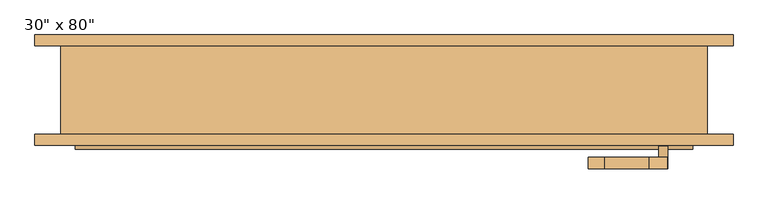
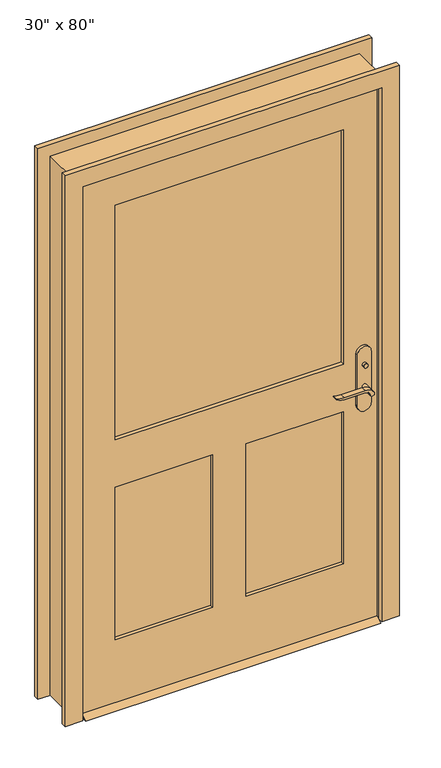
"""IFC4 building model written with IfcOpenShell, lengths in millimetres: door geometry."""

from ifc_helpers import new_model, si_unit, point, frame, frame_2d, origin, place, context, project, spatial, polyline, circle_curve, trimmed, segment, composite_curve, outline, extrude, faceted_brep, source, transform, mapped, element, save


def door_f970b2d0(model_context):
    return source(origin(), model_context, "Body", "SolidModel", [
        extrude(outline(polyline([(-38.1, 12.7), (-12.7, 0.0), (-98.425, 0.0), (-73.025, 12.7), (-38.1, 12.7)])), frame((-533.4, 0.0, 0.0), z_axis=(1.0, 0.0, 0.0), x_axis=(0.0, 1.0, 0.0)), (0.0, 0.0, 1.0), 1066.8),
        extrude(outline(polyline([(487.6, -18.1), (487.6, -28.1), (477.6, -28.1), (477.6, -18.1), (487.6, -18.1)])), frame((0.0, 0.0, 981.9), z_axis=(0.0, 0.0, 1.0), x_axis=(1.0, 0.0, 0.0)), (0.0, 0.0, 1.0), 30.0),
        extrude(outline(composite_curve([segment(trimmed(circle_curve(frame_2d((996.9, 482.6)), 8.0), [point((996.9, 474.6))], [point((996.9, 490.6))], False, "CARTESIAN"), True, "CONTINUOUS"), segment(trimmed(circle_curve(frame_2d((996.9, 482.6)), 8.0), [point((996.9, 490.6))], [point((996.9, 474.6))], False, "CARTESIAN"), True, "CONTINUOUS")], self_intersect=False)), frame((0.0, -93.025, 0.0), z_axis=(0.0, 1.0, 0.0), x_axis=(0.0, 0.0, 1.0)), (0.0, 0.0, 1.0), 10.0),
        extrude(outline(composite_curve([segment(trimmed(circle_curve(frame_2d((897.1555521, 458.9324871)), 37.2832219), [point((919.0523287, 489.1081363))], [point((934.4, 457.2325667))], False, "CARTESIAN"), True, "CONTINUOUS"), segment(polyline([(934.4, 457.2325667), (934.4, 380.9564091)]), True, "CONTINUOUS"), segment(trimmed(circle_curve(frame_2d((1017.6850638, 381.0227909)), 83.2850902), [point((934.4, 380.9564091))], [point((939.4, 352.6))], True, "CARTESIAN"), True, "CONTINUOUS"), segment(polyline([(939.4, 352.6), (936.6135558, 352.6)]), True, "CONTINUOUS"), segment(trimmed(circle_curve(frame_2d((986.6709207, 384.5396612)), 59.3791355), [point((936.6135558, 352.6))], [point((927.4, 380.9564091))], False, "CARTESIAN"), True, "CONTINUOUS"), segment(polyline([(927.4, 380.9564091), (927.4, 457.2138099)]), True, "CONTINUOUS"), segment(trimmed(circle_curve(frame_2d((909.2738613, 457.2138099)), 18.1261387), [point((927.4, 457.2138099))], [point((914.4, 474.6))], True, "CARTESIAN"), True, "CONTINUOUS"), segment(trimmed(circle_curve(frame_2d((914.4, 482.6)), 8.0), [point((914.4, 474.6))], [point((919.0523287, 489.1081363))], False, "CARTESIAN"), True, "CONTINUOUS")], self_intersect=False)), frame((0.0, 1.9, 0.0), z_axis=(0.0, 1.0, 0.0), x_axis=(0.0, 0.0, 1.0)), (0.0, 0.0, 1.0), 20.0),
        extrude(outline(composite_curve([segment(trimmed(circle_curve(frame_2d((914.4, 482.6)), 8.0), [point((914.3999903, 474.6))], [point((919.0523287, 489.1081363))], False, "CARTESIAN"), True, "CONTINUOUS"), segment(trimmed(circle_curve(frame_2d((897.1555521, 458.9324871)), 37.2832219), [point((919.0523287, 489.1081363))], [point((934.4, 457.2325667))], False, "CARTESIAN"), True, "CONTINUOUS"), segment(polyline([(934.4, 457.2325667), (934.4, 380.9564091)]), True, "CONTINUOUS"), segment(trimmed(circle_curve(frame_2d((1017.6850638, 381.0227909)), 83.2850902), [point((934.4, 380.9564091))], [point((939.4, 352.6))], True, "CARTESIAN"), True, "CONTINUOUS"), segment(polyline([(939.4, 352.6), (936.6135558, 352.6)]), True, "CONTINUOUS"), segment(trimmed(circle_curve(frame_2d((986.6709207, 384.5396612)), 59.3791355), [point((936.6135558, 352.6))], [point((927.4, 380.9564091))], False, "CARTESIAN"), True, "CONTINUOUS"), segment(polyline([(927.4, 380.9564091), (927.4, 457.2138122)]), True, "CONTINUOUS"), segment(trimmed(circle_curve(frame_2d((909.2738682, 457.2138122)), 18.1261318), [point((927.4, 457.2138122))], [point((914.3999903, 474.6))], True, "CARTESIAN"), True, "CONTINUOUS")], self_intersect=False)), frame((0.0, -133.025, 0.0), z_axis=(0.0, 1.0, 0.0), x_axis=(0.0, 0.0, 1.0)), (0.0, 0.0, 1.0), 20.0),
        extrude(outline(composite_curve([segment(trimmed(circle_curve(frame_2d((914.4, 482.6)), 8.0), [point((914.4, 474.6))], [point((914.4, 490.6))], False, "CARTESIAN"), True, "CONTINUOUS"), segment(trimmed(circle_curve(frame_2d((914.4, 482.6)), 8.0), [point((914.4, 490.6))], [point((914.4, 474.6))], False, "CARTESIAN"), True, "CONTINUOUS")], self_intersect=False)), frame((0.0, -28.1, 0.0), z_axis=(0.0, 1.0, 0.0), x_axis=(0.0, 0.0, 1.0)), (0.0, 0.0, 1.0), 30.0),
        extrude(outline(composite_curve([segment(trimmed(circle_curve(frame_2d((914.4, 482.6)), 8.0), [point((914.4, 474.6))], [point((914.4, 490.6))], False, "CARTESIAN"), True, "CONTINUOUS"), segment(trimmed(circle_curve(frame_2d((914.4, 482.6)), 8.0), [point((914.4, 490.6))], [point((914.4, 474.6))], False, "CARTESIAN"), True, "CONTINUOUS")], self_intersect=False)), frame((0.0, -113.025, 0.0), z_axis=(0.0, 1.0, 0.0), x_axis=(0.0, 0.0, 1.0)), (0.0, 0.0, 1.0), 30.0),
        extrude(outline(composite_curve([segment(polyline([(844.4, 507.6), (1039.4, 507.6)]), True, "CONTINUOUS"), segment(trimmed(circle_curve(frame_2d((1039.4, 482.6)), 25.0), [point((1039.4, 507.6))], [point((1039.4, 457.6))], False, "CARTESIAN"), True, "CONTINUOUS"), segment(polyline([(1039.4, 457.6), (844.4, 457.6)]), True, "CONTINUOUS"), segment(trimmed(circle_curve(frame_2d((844.4, 482.6)), 25.0), [point((844.4, 457.6))], [point((844.4, 507.6))], False, "CARTESIAN"), True, "CONTINUOUS")], self_intersect=False)), frame((0.0, -38.1, 0.0), z_axis=(0.0, 1.0, 0.0), x_axis=(0.0, 0.0, 1.0)), (0.0, 0.0, 1.0), 10.0),
        extrude(outline(composite_curve([segment(polyline([(844.4, 507.6), (1039.4, 507.6)]), True, "CONTINUOUS"), segment(trimmed(circle_curve(frame_2d((1039.4, 482.6)), 25.0), [point((1039.4, 507.6))], [point((1039.4, 457.6))], False, "CARTESIAN"), True, "CONTINUOUS"), segment(polyline([(1039.4, 457.6), (844.4, 457.6)]), True, "CONTINUOUS"), segment(trimmed(circle_curve(frame_2d((844.4, 482.6)), 25.0), [point((844.4, 457.6))], [point((844.4, 507.6))], False, "CARTESIAN"), True, "CONTINUOUS")], self_intersect=False)), frame((0.0, -83.025, 0.0), z_axis=(0.0, 1.0, 0.0), x_axis=(0.0, 0.0, 1.0)), (0.0, 0.0, 1.0), 10.0),
        extrude(outline(polyline([(2032.0, -533.4), (12.7, -533.4), (12.7, 533.4), (2032.0, 533.4), (2032.0, -533.4)]), holes=[polyline([(1016.0, -412.75), (1911.35, -412.75), (1911.35, 412.75), (1016.0, 412.75), (1016.0, -412.75)]), polyline([(835.025, -60.325), (254.0, -60.325), (254.0, -412.75), (835.025, -412.75), (835.025, -60.325)]), polyline([(835.025, 412.75), (254.0, 412.75), (254.0, 60.325), (835.025, 60.325), (835.025, 412.75)])]), frame((0.0, -73.025, 0.0), z_axis=(0.0, 1.0, 0.0), x_axis=(0.0, 0.0, 1.0)), (0.0, 0.0, 1.0), 34.925),
        faceted_brep([(558.8, -73.025, 0.0), (533.4, -73.025, 0.0), (533.4, -38.1, 0.0), (520.7, -38.1, 0.0), (520.7, -3.175, 0.0), (533.4, -3.175, 0.0), (533.4, 79.375, 0.0), (558.8, 79.375, 0.0), (558.8, 79.375, 2057.4), (558.8, -73.025, 2057.4), (533.4, 79.375, 2032.0), (-533.4, 79.375, 2032.0), (-533.4, 79.375, 0.0), (-558.8, 79.375, 0.0), (-558.8, 79.375, 2057.4), (533.4, -3.175, 2032.0), (520.7, -3.175, 2019.3), (-520.7, -3.175, 2019.3), (-520.7, -3.175, 0.0), (-533.4, -3.175, 0.0), (-533.4, -3.175, 2032.0), (520.7, -38.1, 2019.3), (533.4, -38.1, 2032.0), (-533.4, -38.1, 2032.0), (-533.4, -38.1, 0.0), (-520.7, -38.1, 0.0), (-520.7, -38.1, 2019.3), (533.4, -73.025, 2032.0), (-558.8, -73.025, 2057.4), (-558.8, -73.025, 0.0), (-533.4, -73.025, 0.0), (-533.4, -73.025, 2032.0)], [[[0, 1, 2, 3, 4, 5, 6, 7]], [[7, 8, 9, 0]], [[6, 10, 11, 12, 13, 14, 8, 7]], [[5, 15, 10, 6]], [[4, 16, 17, 18, 19, 20, 15, 5]], [[3, 21, 16, 4]], [[2, 22, 23, 24, 25, 26, 21, 3]], [[1, 27, 22, 2]], [[0, 9, 28, 29, 30, 31, 27, 1]], [[8, 14, 28, 9]], [[15, 20, 11, 10]], [[21, 26, 17, 16]], [[27, 31, 23, 22]], [[29, 13, 12, 19, 18, 25, 24, 30]], [[14, 13, 29, 28]], [[20, 19, 12, 11]], [[26, 25, 18, 17]], [[31, 30, 24, 23]]]),
        extrude(outline(polyline([(-60.325, -49.7416667), (-60.325, -61.3833333), (-412.75, -61.3833333), (-412.75, -49.7416667), (-60.325, -49.7416667)])), frame((0.0, 0.0, 254.0), z_axis=(0.0, 0.0, 1.0), x_axis=(1.0, 0.0, 0.0)), (0.0, 0.0, 1.0), 581.025),
        extrude(outline(polyline([(412.75, -49.7416667), (412.75, -61.3833333), (60.325, -61.3833333), (60.325, -49.7416667), (412.75, -49.7416667)])), frame((0.0, 0.0, 254.0), z_axis=(0.0, 0.0, 1.0), x_axis=(1.0, 0.0, 0.0)), (0.0, 0.0, 1.0), 581.025),
        extrude(outline(polyline([(412.75, -52.07), (412.75, -59.055), (-412.75, -59.055), (-412.75, -52.07), (412.75, -52.07)])), frame((0.0, 0.0, 1016.0), z_axis=(0.0, 0.0, 1.0), x_axis=(1.0, 0.0, 0.0)), (0.0, 0.0, 1.0), 895.35),
        extrude(outline(polyline([(0.0, -539.75), (2038.35, -539.75), (2038.35, 539.75), (0.0, 539.75), (0.0, 603.25), (2101.85, 603.25), (2101.85, -603.25), (0.0, -603.25), (0.0, -539.75)])), frame((0.0, 79.375, 0.0), z_axis=(0.0, 1.0, 0.0), x_axis=(0.0, 0.0, 1.0)), (0.0, 0.0, 1.0), 19.05),
        extrude(outline(polyline([(0.0, -539.75), (2038.35, -539.75), (2038.35, 539.75), (0.0, 539.75), (0.0, 603.25), (2101.85, 603.25), (2101.85, -603.25), (0.0, -603.25), (0.0, -539.75)])), frame((0.0, -92.075, 0.0), z_axis=(0.0, 1.0, 0.0), x_axis=(0.0, 0.0, 1.0)), (0.0, 0.0, 1.0), 19.05),
    ])


if __name__ == "__main__":
    model = new_model("IFC4")
    model_context = context("Model", 3, world=origin())
    ifc_project = project(units=[si_unit("LENGTHUNIT", "METRE", prefix="MILLI")], contexts=[model_context])
    site = spatial("IfcSite", under=ifc_project)
    building = spatial("IfcBuilding", under=site)
    placement = place(None, origin())
    door_shape = door_f970b2d0(model_context)
    element("IfcDoor", 1, ObjectType="30\" x 80\"", at=placement, inside=building, context=model_context, shape_type="MappedRepresentation", body=[
        mapped(door_shape, transform((0.0, 0.0, 0.0), x_axis=(1.0, 0.0, 0.0), y_axis=(0.0, 1.0, 0.0), z_axis=(0.0, 0.0, 1.0))),
    ])
    save(model, "model.ifc")

# Revit data of these elements
# Type "30\" x 80\""
#   Type Mark = "11"
#   Assembly Code = "B2030100"
#   Analytic Construction = "French door, wood frame with single glass"
#   Top Rail = 0' - 4 3/4"
#   Threshold Offset [instance default] = 0' - 0 1/2"
#   Thickness = 0' - 1 3/8"
#   Thermal Resistance (R) = 1.0696 (h·ft²·°F)/BTU
#   Swing Angle [instance default] = 90.00°
#   Stiles = 0' - 4 3/4"
#   Rough Width = 3' - 8"
#   Rough Height = 6' - 9"
#   Lock Rail = 0' - 7 1/8"
#   Height = 6' - 8"
#   Width = 3' - 6"
#   Heat Transfer Coefficient (U) = 0.9350 BTU/(h·ft²·°F)
#   Door Offset [instance default] = 0' - 0"
#   Bottom Rail = 0' - 9 1/2"
#   Threshold [instance default] = yes
#   Function = 1
#   Exterior Trim [instance default] = yes
#   Trim Material = Cherry
#   Threshold Material = Cherry
#   Panel Material = Cherry
#   Glazing = Glass
#   Frame Material = Cherry
#   Door Handle Material = Aluminum
#   Visual Light Transmittance = 0
#   Solar Heat Gain Coefficient = 0
#   Wall Closure = (empty or 0)
#   Construction Type = (empty or 0)
# Element 1 (IfcDoor, "30\" x 80\"")
#   Materials on its faces: "Cherry", "Aluminum", "Glass"
# Materials
#   "Cherry": class "Wood", colour RGB 226 177 128, transparency 0, Description = "Prunus Serotina", Cost = 0
#   "Glass": class "Glass", colour RGB 0 128 192, transparency 0.75, Description = "Soda Lime Glass", Cost = 0
#   "Aluminum": class "Metal", colour RGB 247 247 247, transparency 0, Description = "Aluminum 6061", Cost = 0
